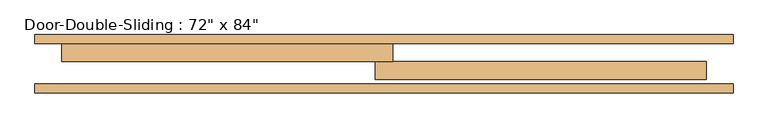
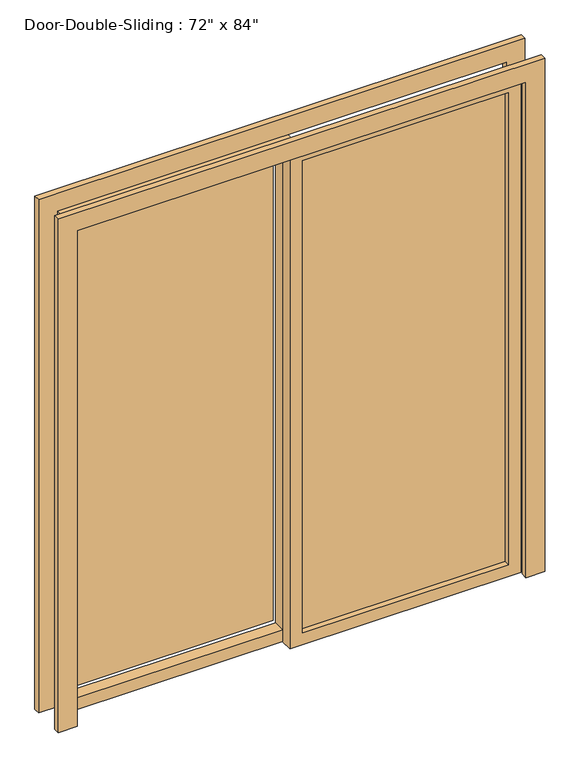
"""IFC4 building model written with IfcOpenShell, lengths in millimetres: door geometry."""

from ifc_helpers import new_model, si_unit, frame, origin, place, context, project, spatial, polyline, outline, extrude, source, transform, mapped, element, save


def door_166d4031(model_context):
    return source(origin(), model_context, "Body", "SweptSolid", [
        extrude(outline(polyline([(0.0, 990.6), (2209.8, 990.6), (2209.8, -990.6), (0.0, -990.6), (0.0, -914.4), (2133.6, -914.4), (2133.6, 914.4), (0.0, 914.4), (0.0, 990.6)])), frame((0.0, 184.15, 0.0), z_axis=(0.0, 1.0, 0.0), x_axis=(0.0, 0.0, 1.0)), (0.0, 0.0, 1.0), 25.4),
        extrude(outline(polyline([(0.0, -990.6), (0.0, -914.4), (2133.6, -914.4), (2133.6, 914.4), (0.0, 914.4), (0.0, 990.6), (2209.8, 990.6), (2209.8, -990.6), (0.0, -990.6)])), frame((0.0, 44.45, 0.0), z_axis=(0.0, 1.0, 0.0), x_axis=(0.0, 0.0, 1.0)), (0.0, 0.0, 1.0), 25.4),
        extrude(outline(polyline([(2133.6, 25.4), (2133.6, -914.4), (0.0, -914.4), (0.0, 25.4), (2133.6, 25.4)]), holes=[polyline([(2082.8, -25.4), (50.8, -25.4), (50.8, -863.6), (2082.8, -863.6), (2082.8, -25.4)])]), frame((0.0, 133.35, 0.0), z_axis=(0.0, 1.0, 0.0), x_axis=(0.0, 0.0, 1.0)), (0.0, 0.0, 1.0), 50.8),
        extrude(outline(polyline([(2133.6, -25.4), (0.0, -25.4), (0.0, 914.4), (2133.6, 914.4), (2133.6, -25.4)]), holes=[polyline([(2082.8, 25.4), (2082.8, 863.6), (50.8, 863.6), (50.8, 25.4), (2082.8, 25.4)])]), frame((0.0, 82.55, 0.0), z_axis=(0.0, 1.0, 0.0), x_axis=(0.0, 0.0, 1.0)), (0.0, 0.0, 1.0), 50.8),
        extrude(outline(polyline([(-25.4, 200.025), (-863.6, 200.025), (-863.6, 206.375), (-25.4, 206.375), (-25.4, 200.025)])), frame((0.0, 0.0, 50.8), z_axis=(0.0, 0.0, 1.0), x_axis=(1.0, 0.0, 0.0)), (0.0, 0.0, 1.0), 2032.0),
        extrude(outline(polyline([(25.4, 111.125), (863.6, 111.125), (863.6, 104.775), (25.4, 104.775), (25.4, 111.125)])), frame((0.0, 0.0, 50.8), z_axis=(0.0, 0.0, 1.0), x_axis=(1.0, 0.0, 0.0)), (0.0, 0.0, 1.0), 2032.0),
    ])


if __name__ == "__main__":
    model = new_model("IFC4")
    model_context = context("Model", 3, world=origin())
    ifc_project = project(units=[si_unit("LENGTHUNIT", "METRE", prefix="MILLI")], contexts=[model_context])
    site = spatial("IfcSite", under=ifc_project)
    building = spatial("IfcBuilding", under=site)
    placement = place(None, origin())
    door_shape = door_166d4031(model_context)
    element("IfcDoor", 1, ObjectType="Door-Double-Sliding : 72\" x 84\"", at=placement, inside=building, context=model_context, shape_type="MappedRepresentation", body=[
        mapped(door_shape, transform((0.0, 0.0, 0.0), x_axis=(1.0, 0.0, 0.0), y_axis=(0.0, 1.0, 0.0), z_axis=(0.0, 0.0, 1.0))),
    ])
    save(model, "model.ifc")

# Revit data of these elements
# Type "Door-Double-Sliding : 72\" x 84\""
#   Type Mark = "8"
#   Construction Type Id = "opn-d45"
#   Assembly Code = "C1020"
#   Analytic Construction = "Wood frame, double glass door "
#   Thickness = 0' - 2"
#   Thermal Resistance (R) = 1.8150 (h·ft²·°F)/BTU
#   Heat Transfer Coefficient (U) = 0.5510 BTU/(h·ft²·°F)
#   Height = 7' - 0"
#   Rail Width = 0' - 2"
#   Stiles = 0' - 2"
#   Trim Projection Ext = 0' - 1"
#   Trim Projection Int = 0' - 1"
#   Trim Width = 0' - 3"
#   Width = 6' - 0"
#   Define Thermal Properties by = 1
#   Glazing = Glass
#   Panel Material = Wood - Birch - Solid Stained Light Low Gloss
#   Trim Material = Paint - Sienna
#   Visual Light Transmittance = 0
#   Solar Heat Gain Coefficient = 0
#   Function = (empty or 0)
#   Wall Closure = (empty or 0)
# Element 1 (IfcDoor, "Door-Double-Sliding : 72\" x 84\"")
#   Materials on its faces: "Paint - Sienna", "Wood - Birch - Solid Stained Light Low Gloss", "Glass"
# Materials
#   "Glass": class "Glass", colour RGB 0 128 192, transparency 0.75, Description = "Soda Lime Glass", Cost = 0
#   "Wood - Birch - Solid Stained Light Low Gloss": class "Wood", colour RGB 210 159 95, transparency 0, Cost = 0
#   "Paint - Sienna": colour RGB 118 70 51, transparency 0, Cost = 0
